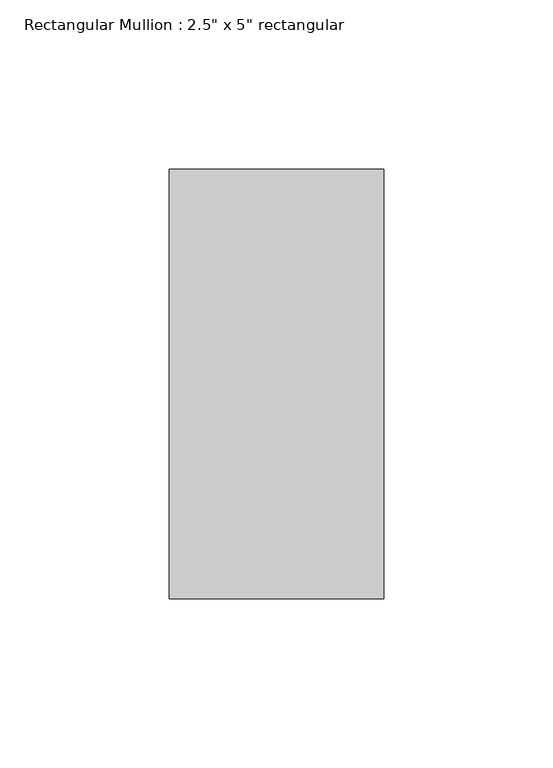
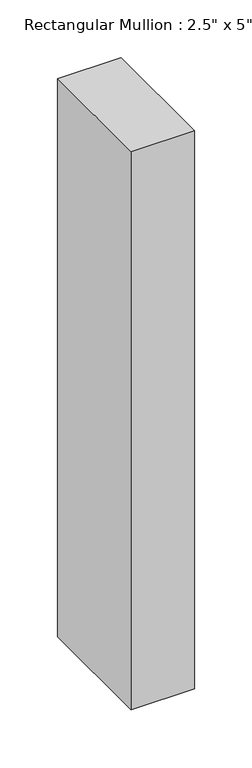
"""IFC4 building model written with IfcOpenShell, lengths in millimetres: member geometry."""

from ifc_helpers import new_model, si_unit, frame, origin, place, context, project, spatial, polyline, outline, extrude, source, transform, mapped, element, save


def member_29dce480(model_context):
    return source(origin(), model_context, "Body", "SweptSolid", [
        extrude(outline(polyline([(31.75, 63.5), (31.75, -63.5), (-31.75, -63.5), (-31.75, 63.5), (31.75, 63.5)])), frame((0.0, 0.0, -590.55), z_axis=(0.0, 0.0, 1.0), x_axis=(1.0, 0.0, 0.0)), (0.0, 0.0, 1.0), 590.55),
    ])


if __name__ == "__main__":
    model = new_model("IFC4")
    model_context = context("Model", 3, world=origin())
    ifc_project = project(units=[si_unit("LENGTHUNIT", "METRE", prefix="MILLI")], contexts=[model_context])
    site = spatial("IfcSite", under=ifc_project)
    building = spatial("IfcBuilding", under=site)
    placement = place(None, origin())
    member_shape = member_29dce480(model_context)
    element("IfcMember", 1, ObjectType="Rectangular Mullion : 2.5\" x 5\" rectangular", at=placement, inside=building, context=model_context, shape_type="MappedRepresentation", body=[
        mapped(member_shape, transform((0.0, 0.0, 0.0), x_axis=(1.0, 0.0, 0.0), y_axis=(0.0, 1.0, 0.0), z_axis=(0.0, 0.0, 1.0))),
    ])
    save(model, "model.ifc")

# Revit data of these elements
# Type "Rectangular Mullion : 2.5\" x 5\" rectangular"
#   built-in parameter 1007304 = 0.416667 (stored number, unit not read)
#   built-in parameter 1007301 = 0.104167 (stored number, unit not read)
#   built-in parameter 1007300 = 0.104167 (stored number, unit not read)
# Element 1 (IfcMember, "Rectangular Mullion : 2.5\" x 5\" rectangular")
#   Materials on its faces: "Aluminum"
# Materials
#   "Aluminum": class "Metal", colour RGB 247 247 247, transparency 0, Description = "Aluminum 6061", Cost = 0
